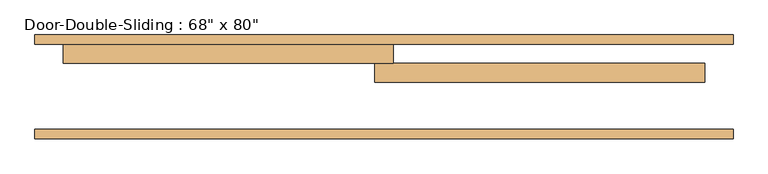
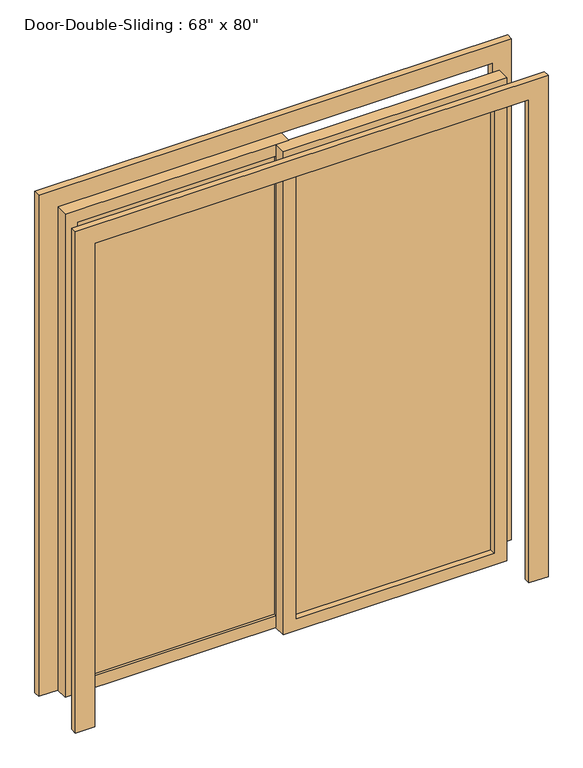
"""IFC4 building model written with IfcOpenShell, lengths in millimetres: door geometry."""

from ifc_helpers import new_model, si_unit, frame, origin, place, context, project, spatial, polyline, outline, extrude, source, transform, mapped, element, save


def door_ed3b37b7(model_context):
    return source(origin(), model_context, "Body", "SweptSolid", [
        extrude(outline(polyline([(0.0, 939.8), (2108.2, 939.8), (2108.2, -939.8), (0.0, -939.8), (0.0, -863.6), (2032.0, -863.6), (2032.0, 863.6), (0.0, 863.6), (0.0, 939.8)])), frame((0.0, 241.3, 0.0), z_axis=(0.0, 1.0, 0.0), x_axis=(0.0, 0.0, 1.0)), (0.0, 0.0, 1.0), 25.4),
        extrude(outline(polyline([(0.0, -939.8), (0.0, -863.6), (2032.0, -863.6), (2032.0, 863.6), (0.0, 863.6), (0.0, 939.8), (2108.2, 939.8), (2108.2, -939.8), (0.0, -939.8)])), frame((0.0, -12.7, 0.0), z_axis=(0.0, 1.0, 0.0), x_axis=(0.0, 0.0, 1.0)), (0.0, 0.0, 1.0), 25.4),
        extrude(outline(polyline([(2032.0, 25.4), (2032.0, -863.6), (0.0, -863.6), (0.0, 25.4), (2032.0, 25.4)]), holes=[polyline([(1981.2, -25.4), (50.8, -25.4), (50.8, -812.8), (1981.2, -812.8), (1981.2, -25.4)])]), frame((0.0, 190.5, 0.0), z_axis=(0.0, 1.0, 0.0), x_axis=(0.0, 0.0, 1.0)), (0.0, 0.0, 1.0), 50.8),
        extrude(outline(polyline([(2032.0, -25.4), (0.0, -25.4), (0.0, 863.6), (2032.0, 863.6), (2032.0, -25.4)]), holes=[polyline([(1981.2, 25.4), (1981.2, 812.8), (50.8, 812.8), (50.8, 25.4), (1981.2, 25.4)])]), frame((0.0, 139.7, 0.0), z_axis=(0.0, 1.0, 0.0), x_axis=(0.0, 0.0, 1.0)), (0.0, 0.0, 1.0), 50.8),
        extrude(outline(polyline([(-25.4, 200.025), (-812.8, 200.025), (-812.8, 206.375), (-25.4, 206.375), (-25.4, 200.025)])), frame((0.0, 0.0, 50.8), z_axis=(0.0, 0.0, 1.0), x_axis=(1.0, 0.0, 0.0)), (0.0, 0.0, 1.0), 1930.4),
        extrude(outline(polyline([(25.4, 168.275), (812.8, 168.275), (812.8, 161.925), (25.4, 161.925), (25.4, 168.275)])), frame((0.0, 0.0, 50.8), z_axis=(0.0, 0.0, 1.0), x_axis=(1.0, 0.0, 0.0)), (0.0, 0.0, 1.0), 1930.4),
    ])


if __name__ == "__main__":
    model = new_model("IFC4")
    model_context = context("Model", 3, world=origin())
    ifc_project = project(units=[si_unit("LENGTHUNIT", "METRE", prefix="MILLI")], contexts=[model_context])
    site = spatial("IfcSite", under=ifc_project)
    building = spatial("IfcBuilding", under=site)
    placement = place(None, origin())
    door_shape = door_ed3b37b7(model_context)
    element("IfcDoor", 1, ObjectType="Door-Double-Sliding : 68\" x 80\"", at=placement, inside=building, context=model_context, shape_type="MappedRepresentation", body=[
        mapped(door_shape, transform((0.0, 0.0, 0.0), x_axis=(1.0, 0.0, 0.0), y_axis=(0.0, 1.0, 0.0), z_axis=(0.0, 0.0, 1.0))),
    ])
    save(model, "model.ifc")

# Revit data of these elements
# Type "Door-Double-Sliding : 68\" x 80\""
#   Type Mark = "10"
#   Construction Type Id = "opn-d45"
#   Assembly Code = "C1020"
#   Analytic Construction = "Wood frame, double glass door "
#   Thickness = 0' - 2"
#   Thermal Resistance (R) = 1.8150 (h·ft²·°F)/BTU
#   Heat Transfer Coefficient (U) = 0.5510 BTU/(h·ft²·°F)
#   Height = 6' - 8"
#   Rail Width = 0' - 2"
#   Stiles = 0' - 2"
#   Trim Projection Ext = 0' - 1"
#   Trim Projection Int = 0' - 1"
#   Trim Width = 0' - 3"
#   Width = 5' - 8"
#   Define Thermal Properties by = 1
#   Glazing = Glass
#   Panel Material = Wood - Birch - Solid Stained Light Low Gloss
#   Trim Material = Paint - Sienna
#   Visual Light Transmittance = 0
#   Solar Heat Gain Coefficient = 0
#   Function = (empty or 0)
#   Wall Closure = (empty or 0)
# Element 1 (IfcDoor, "Door-Double-Sliding : 68\" x 80\"")
#   Materials on its faces: "Paint - Sienna", "Wood - Birch - Solid Stained Light Low Gloss", "Glass"
# Materials
#   "Glass": class "Glass", colour RGB 0 128 192, transparency 0.75, Description = "Soda Lime Glass", Cost = 0
#   "Wood - Birch - Solid Stained Light Low Gloss": class "Wood", colour RGB 210 159 95, transparency 0, Cost = 0
#   "Paint - Sienna": colour RGB 118 70 51, transparency 0, Cost = 0
